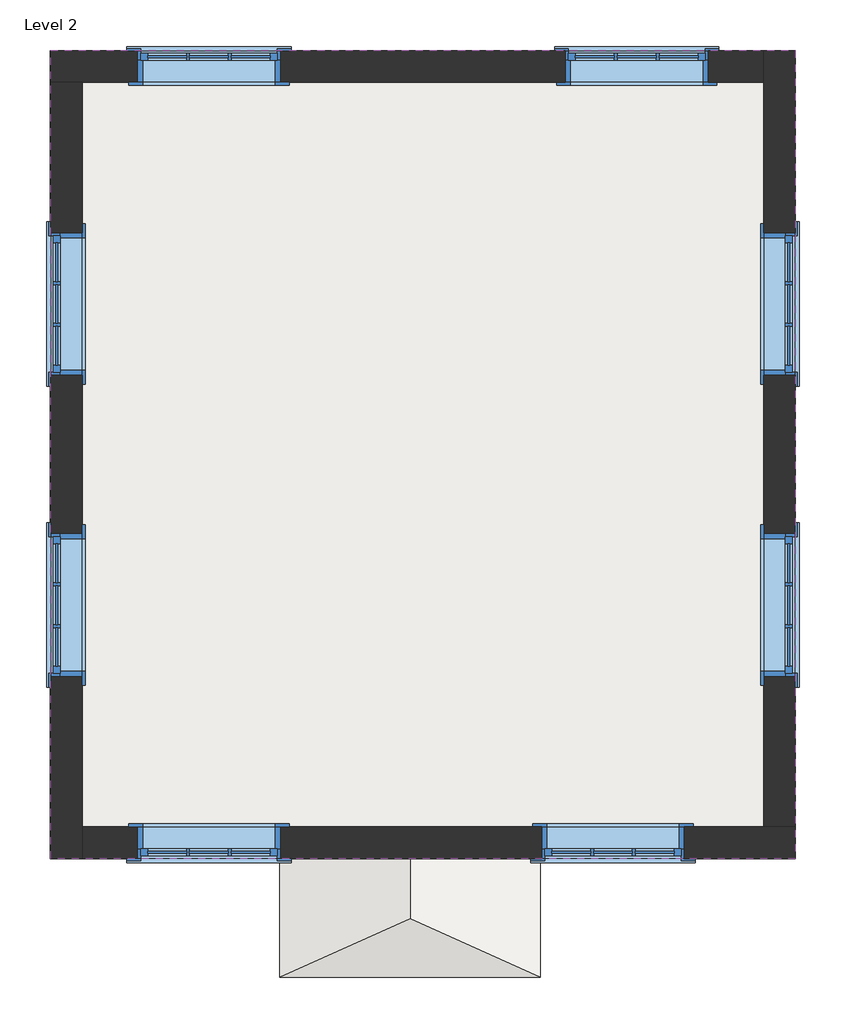
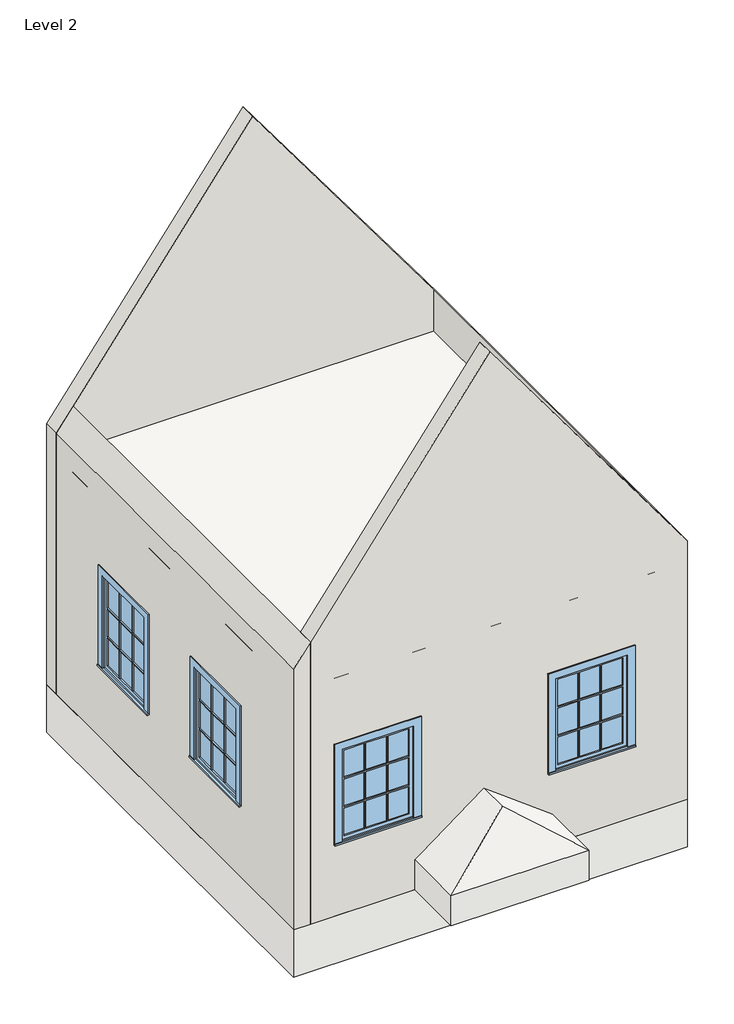
# One storey: 8 windows, 4 walls, 2 slabs, 1 roof.
"""IFC4 building model written with IfcOpenShell, lengths in millimetres."""

from ifc_helpers import new_model, si_unit, frame, origin, place, context, project, spatial, polyline, outline, extrude, faceted_brep, transform, mapped, element, save
from components import window_29c06734

model = new_model("IFC4")

# Units and contexts
model_context = context("Model", 3, world=origin())
ifc_project = project(units=[si_unit("LENGTHUNIT", "METRE", prefix="MILLI")], contexts=[model_context])

# Site, building, storey
site = spatial("IfcSite", under=ifc_project)
building = spatial("IfcBuilding", under=site)
storey = spatial("IfcBuildingStorey", under=building, Name="Level 2", Elevation=3048.0)

# Roof
placement = place(None, origin())
element("IfcRoof", 1, ObjectType="Generic - 12\"", at=placement, inside=storey, context=model_context, shape_type="Brep", body=[
    faceted_brep([(-8140.4670776, -8162.062689, 3048.0), (-8140.4670776, -7527.3100774, 3048.0), (-7305.4420776, -7527.3100774, 3674.26875), (-7305.4420776, -7787.3972655, 3674.26875), (-6470.4170776, -8162.062689, 3048.0), (-6470.4170776, -7527.3100774, 3048.0), (-8140.4670776, -7527.3100774, 3429.0), (-8140.4670776, -8289.3100774, 3429.0), (-7305.4420776, -7914.644654, 4055.26875), (-7305.4420776, -7527.3100774, 4055.26875), (-6470.4170776, -8289.3100774, 3429.0), (-6470.4170776, -7527.3100774, 3429.0), (-8140.4670776, -8289.3100774, 3048.0), (-6470.4170776, -8289.3100774, 3048.0)], [[[0, 1, 2, 3]], [[0, 3, 4]], [[5, 4, 3, 2]], [[6, 7, 8, 9]], [[7, 10, 8]], [[11, 9, 8, 10]], [[12, 7, 6, 1, 0]], [[13, 10, 7, 12]], [[5, 11, 10, 13, 4]], [[4, 13, 12, 0]], [[6, 9, 11, 5, 2, 1]]]),
])

# Slabs
element("IfcSlab", 2, ObjectType="Generic - 12\"", at=placement, inside=storey, context=model_context, shape_type="SweptSolid", body=[
    extrude(outline(polyline([(-9613.6670776, -7527.3100774), (-9613.6670776, -2345.7100774), (-4838.4670776, -2345.7100774), (-4838.4670776, -7527.3100774), (-9613.6670776, -7527.3100774)])), frame((0.0, 0.0, 2438.4), z_axis=(0.0, 0.0, 1.0), x_axis=(1.0, 0.0, 0.0)), (0.0, 0.0, 1.0), 609.6),
])
element("IfcSlab", 3, ObjectType="Generic - 12\"", at=placement, inside=storey, context=model_context, shape_type="SweptSolid", body=[
    extrude(outline(polyline([(-9610.8300594, -7527.3100774), (-9610.8300594, -2345.7100774), (-4835.6300594, -2345.7100774), (-4835.6300594, -7527.3100774), (-9610.8300594, -7527.3100774)])), frame((0.0, 0.0, 5486.4), z_axis=(0.0, 0.0, 1.0), x_axis=(1.0, 0.0, 0.0)), (0.0, 0.0, 1.0), 609.6),
])

# Walls
element("IfcWall", 4, ObjectType="Generic - 8\"", at=placement, inside=storey, context=model_context, shape_type="Brep", body=[
    faceted_brep([(-9610.8300594, -2548.9100774, 3048.0), (-9407.6300594, -2548.9100774, 3048.0), (-5038.8300594, -2548.9100774, 3048.0), (-5038.8300594, -2548.9100774, 6634.6074998), (-7233.256206, -2548.9100774, 9616.4751741), (-9407.6300594, -2548.9100774, 6661.8552999), (-9610.8300594, -2548.9100774, 6385.7396), (-5394.4300594, -2548.9100774, 5181.6), (-5394.4300594, -2548.9100774, 3962.4), (-6308.8300594, -2548.9100774, 3962.4), (-6308.8300594, -2548.9100774, 5181.6), (-8137.6300594, -2548.9100774, 5181.6), (-8137.6300594, -2548.9100774, 3962.4), (-9052.0300594, -2548.9100774, 3962.4), (-9052.0300594, -2548.9100774, 5181.6), (-9610.8300594, -2345.7100774, 3048.0), (-9610.8300594, -2345.7100774, 6385.7396), (-7233.256206, -2345.7100774, 9616.4751741), (-5038.8300594, -2345.7100774, 6634.6074998), (-5038.8300594, -2345.7100774, 3048.0), (-5394.4300594, -2345.7100774, 5181.6), (-6308.8300594, -2345.7100774, 5181.6), (-6308.8300594, -2345.7100774, 3962.4), (-5394.4300594, -2345.7100774, 3962.4), (-8137.6300594, -2345.7100774, 5181.6), (-9052.0300594, -2345.7100774, 5181.6), (-9052.0300594, -2345.7100774, 3962.4), (-8137.6300594, -2345.7100774, 3962.4)], [[[0, 1, 2, 3, 4, 5, 6], [7, 8, 9, 10], [11, 12, 13, 14]], [[15, 16, 17, 18, 19], [20, 21, 22, 23], [24, 25, 26, 27]], [[2, 1, 0, 15, 19]], [[0, 6, 16, 15]], [[3, 2, 19, 18]], [[8, 7, 20, 23]], [[9, 8, 23, 22]], [[10, 9, 22, 21]], [[7, 10, 21, 20]], [[12, 11, 24, 27]], [[13, 12, 27, 26]], [[14, 13, 26, 25]], [[11, 14, 25, 24]], [[6, 5, 4, 17, 16]], [[4, 3, 18, 17]]]),
])
element("IfcWall", 5, ObjectType="Generic - 8\"", at=placement, inside=storey, context=model_context, shape_type="Brep", body=[
    faceted_brep([(-9407.6300594, -7527.3100774, 3048.0), (-9407.6300594, -7324.1100774, 3048.0), (-9407.6300594, -2548.9100774, 3048.0), (-9407.6300594, -2548.9100774, 6661.8552999), (-9407.6300594, -7324.1100774, 6661.8552999), (-9407.6300594, -7527.3100774, 6661.8552999), (-9407.6300594, -3514.1100774, 5181.6), (-9407.6300594, -3514.1100774, 3962.4), (-9407.6300594, -4428.5100774, 3962.4), (-9407.6300594, -4428.5100774, 5181.6), (-9407.6300594, -5444.5100774, 5181.6), (-9407.6300594, -5444.5100774, 3962.4), (-9407.6300594, -6358.9100774, 3962.4), (-9407.6300594, -6358.9100774, 5181.6), (-9610.8300594, -7527.3100774, 3048.0), (-9610.8300594, -7527.3100774, 6385.7396), (-9610.8300594, -2548.9100774, 6385.7396), (-9610.8300594, -2548.9100774, 3048.0), (-9610.8300594, -3514.1100774, 5181.6), (-9610.8300594, -4428.5100774, 5181.6), (-9610.8300594, -4428.5100774, 3962.4), (-9610.8300594, -3514.1100774, 3962.4), (-9610.8300594, -5444.5100774, 5181.6), (-9610.8300594, -6358.9100774, 5181.6), (-9610.8300594, -6358.9100774, 3962.4), (-9610.8300594, -5444.5100774, 3962.4)], [[[0, 1, 2, 3, 4, 5], [6, 7, 8, 9], [10, 11, 12, 13]], [[14, 15, 16, 17], [18, 19, 20, 21], [22, 23, 24, 25]], [[2, 1, 0, 14, 17]], [[0, 5, 15, 14]], [[3, 2, 17, 16]], [[7, 6, 18, 21]], [[8, 7, 21, 20]], [[9, 8, 20, 19]], [[6, 9, 19, 18]], [[11, 10, 22, 25]], [[12, 11, 25, 24]], [[13, 12, 24, 23]], [[10, 13, 23, 22]], [[5, 4, 3, 16, 15]]]),
])
element("IfcWall", 6, ObjectType="Generic - 8\"", at=placement, inside=storey, context=model_context, shape_type="Brep", body=[
    faceted_brep([(-4835.6300594, -7324.1100774, 3048.0), (-5038.8300594, -7324.1100774, 3048.0), (-9407.6300594, -7324.1100774, 3048.0), (-9407.6300594, -7324.1100774, 6661.8552999), (-7233.256206, -7324.1100774, 9616.4751741), (-5038.8300594, -7324.1100774, 6634.6074998), (-4835.6300594, -7324.1100774, 6358.4917998), (-6461.2300594, -7324.1100774, 5181.6), (-6461.2300594, -7324.1100774, 3962.4), (-5546.8300594, -7324.1100774, 3962.4), (-5546.8300594, -7324.1100774, 5181.6), (-9052.0300594, -7324.1100774, 5181.6), (-9052.0300594, -7324.1100774, 3962.4), (-8137.6300594, -7324.1100774, 3962.4), (-8137.6300594, -7324.1100774, 5181.6), (-4835.6300594, -7527.3100774, 3048.0), (-4835.6300594, -7527.3100774, 6358.4917998), (-7233.256206, -7527.3100774, 9616.4751741), (-9407.6300594, -7527.3100774, 6661.8552999), (-9407.6300594, -7527.3100774, 3048.0), (-6461.2300594, -7527.3100774, 5181.6), (-5546.8300594, -7527.3100774, 5181.6), (-5546.8300594, -7527.3100774, 3962.4), (-6461.2300594, -7527.3100774, 3962.4), (-9052.0300594, -7527.3100774, 5181.6), (-8137.6300594, -7527.3100774, 5181.6), (-8137.6300594, -7527.3100774, 3962.4), (-9052.0300594, -7527.3100774, 3962.4)], [[[0, 1, 2, 3, 4, 5, 6], [7, 8, 9, 10], [11, 12, 13, 14]], [[15, 16, 17, 18, 19], [20, 21, 22, 23], [24, 25, 26, 27]], [[2, 1, 0, 15, 19]], [[0, 6, 16, 15]], [[3, 2, 19, 18]], [[8, 7, 20, 23]], [[9, 8, 23, 22]], [[10, 9, 22, 21]], [[7, 10, 21, 20]], [[12, 11, 24, 27]], [[13, 12, 27, 26]], [[14, 13, 26, 25]], [[11, 14, 25, 24]], [[4, 3, 18, 17]], [[6, 5, 4, 17, 16]]]),
])
element("IfcWall", 7, ObjectType="Generic - 8\"", at=placement, inside=storey, context=model_context, shape_type="Brep", body=[
    faceted_brep([(-5038.8300594, -2345.7100774, 3048.0), (-5038.8300594, -2548.9100774, 3048.0), (-5038.8300594, -7324.1100774, 3048.0), (-5038.8300594, -7324.1100774, 6634.6074998), (-5038.8300594, -2548.9100774, 6634.6074998), (-5038.8300594, -2345.7100774, 6634.6074998), (-5038.8300594, -6358.9100774, 5181.6), (-5038.8300594, -6358.9100774, 3962.4), (-5038.8300594, -5444.5100774, 3962.4), (-5038.8300594, -5444.5100774, 5181.6), (-5038.8300594, -4428.5100774, 5181.6), (-5038.8300594, -4428.5100774, 3962.4), (-5038.8300594, -3514.1100774, 3962.4), (-5038.8300594, -3514.1100774, 5181.6), (-4835.6300594, -2345.7100774, 3048.0), (-4835.6300594, -2345.7100774, 6358.4917998), (-4835.6300594, -7324.1100774, 6358.4917998), (-4835.6300594, -7324.1100774, 3048.0), (-4835.6300594, -6358.9100774, 5181.6), (-4835.6300594, -5444.5100774, 5181.6), (-4835.6300594, -5444.5100774, 3962.4), (-4835.6300594, -6358.9100774, 3962.4), (-4835.6300594, -4428.5100774, 5181.6), (-4835.6300594, -3514.1100774, 5181.6), (-4835.6300594, -3514.1100774, 3962.4), (-4835.6300594, -4428.5100774, 3962.4)], [[[0, 1, 2, 3, 4, 5], [6, 7, 8, 9], [10, 11, 12, 13]], [[14, 15, 16, 17], [18, 19, 20, 21], [22, 23, 24, 25]], [[2, 1, 0, 14, 17]], [[0, 5, 15, 14]], [[3, 2, 17, 16]], [[7, 6, 18, 21]], [[8, 7, 21, 20]], [[9, 8, 20, 19]], [[6, 9, 19, 18]], [[11, 10, 22, 25]], [[12, 11, 25, 24]], [[13, 12, 24, 23]], [[10, 13, 23, 22]], [[5, 4, 3, 16, 15]]]),
])

# Windows
window_shape = window_29c06734(model_context)
element("IfcWindow", 8, ObjectType="Casement 3x3 with Trim : 36\" x 48\"", at=placement, inside=storey, context=model_context, shape_type="MappedRepresentation", body=[
    mapped(window_shape, transform((-4937.2300594, -5901.7100774, 3048.0), x_axis=(0.0, -1.0, 0.0), y_axis=(1.0, 0.0, 0.0), z_axis=(0.0, 0.0, 1.0))),
])
element("IfcWindow", 9, ObjectType="Casement 3x3 with Trim : 36\" x 48\"", at=placement, inside=storey, context=model_context, shape_type="MappedRepresentation", body=[
    mapped(window_shape, transform((-4937.2300594, -3971.3100774, 3048.0), x_axis=(0.0, -1.0, 0.0), y_axis=(1.0, 0.0, 0.0), z_axis=(0.0, 0.0, 1.0))),
])
element("IfcWindow", 10, ObjectType="Casement 3x3 with Trim : 36\" x 48\"", at=placement, inside=storey, context=model_context, shape_type="MappedRepresentation", body=[
    mapped(window_shape, transform((-6004.0300594, -7425.7100774, 3048.0), x_axis=(-1.0, 0.0, 0.0), y_axis=(0.0, -1.0, 0.0), z_axis=(0.0, 0.0, 1.0))),
])
element("IfcWindow", 11, ObjectType="Casement 3x3 with Trim : 36\" x 48\"", at=placement, inside=storey, context=model_context, shape_type="MappedRepresentation", body=[
    mapped(window_shape, transform((-8594.8300594, -7425.7100774, 3048.0), x_axis=(-1.0, 0.0, 0.0), y_axis=(0.0, -1.0, 0.0), z_axis=(0.0, 0.0, 1.0))),
])
element("IfcWindow", 12, ObjectType="Casement 3x3 with Trim : 36\" x 48\"", at=placement, inside=storey, context=model_context, shape_type="MappedRepresentation", body=[
    mapped(window_shape, transform((-9509.2300594, -3971.3100774, 3048.0), x_axis=(0.0, 1.0, 0.0), y_axis=(-1.0, 0.0, 0.0), z_axis=(0.0, 0.0, 1.0))),
])
element("IfcWindow", 13, ObjectType="Casement 3x3 with Trim : 36\" x 48\"", at=placement, inside=storey, context=model_context, shape_type="MappedRepresentation", body=[
    mapped(window_shape, transform((-9509.2300594, -5901.7100774, 3048.0), x_axis=(0.0, 1.0, 0.0), y_axis=(-1.0, 0.0, 0.0), z_axis=(0.0, 0.0, 1.0))),
])
element("IfcWindow", 14, ObjectType="Casement 3x3 with Trim : 36\" x 48\"", at=placement, inside=storey, context=model_context, shape_type="MappedRepresentation", body=[
    mapped(window_shape, transform((-5851.6300594, -2447.3100774, 3048.0), x_axis=(1.0, 0.0, 0.0), y_axis=(0.0, 1.0, 0.0), z_axis=(0.0, 0.0, 1.0))),
])
element("IfcWindow", 15, ObjectType="Casement 3x3 with Trim : 36\" x 48\"", at=placement, inside=storey, context=model_context, shape_type="MappedRepresentation", body=[
    mapped(window_shape, transform((-8594.8300594, -2447.3100774, 3048.0), x_axis=(1.0, 0.0, 0.0), y_axis=(0.0, 1.0, 0.0), z_axis=(0.0, 0.0, 1.0))),
])

save(model, "model.ifc")

# Revit data of these elements
# Type "Generic - 12\""
#   Assembly Code = "B1020"
#   Layers, outside or top first: 1' - 0" no material (function 1)
# Type "Generic - 12\""
#   Assembly Code = "B1010"
#   Function = 0
#   Layers, outside or top first: 2' - 0" no material (function 1)
# Type "Generic - 8\""
#   Assembly Code = "B2010"
#   Layers, outside or top first: 0' - 8" no material (function 1)
# Type "Casement 3x3 with Trim : 36\" x 48\""
#   Type Mark = "10"
#   Construction Type Id = "GSP4R"
#   Assembly Code = "B2020100"
#   Analytic Construction = "1/8 in Pilkington single glazing"
#   Visual Light Transmittance = 0.9
#   Solar Heat Gain Coefficient = 0.78
#   Heat Transfer Coefficient (U) = 0.6496 BTU/(h·ft²·°F)
#   Height = 4' - 0"
#   Default Sill Height = 3' - 0"
#   Trim Projection - Ext. = 0' - 0 1/2"
#   Trim Projection - Int. = 0' - 0 3/4"
#   Trim Width - Exterior = 0' - 3 1/2"
#   Trim Width - Interior = 0' - 3 1/2"
#   Width = 3' - 0"
#   Window Inset = 0' - 0 3/4"
#   Define Thermal Properties by = 1
#   Glass Pane Material = Glass
#   Sash Material = Sash
#   Trim Exterior Material = Trim
#   Trim Interior Material = Trim
#   Wall Closure = (empty or 0)
# Element 1 (IfcRoof, "Generic - 12\"")
#   built-in parameter 1001705 = 13.3047 (stored number, unit not read)
#   built-in parameter 1001710 = 33615
#   Phase Created = New Construction
#   Materials on its faces: "Default Roof"
# Element 2 (IfcSlab, "Generic - 12\"")
#   built-in parameter 1001955 = 3.14159 (stored number, unit not read)
#   Height Offset From Level = 0' - 0"
#   Phase Created = New Construction
#   Materials on its faces: "Default Floor"
# Element 3 (IfcSlab, "Generic - 12\"")
#   built-in parameter 1001955 = 3.14159 (stored number, unit not read)
#   Height Offset From Level = 10' - 0"
#   Phase Created = New Construction
#   Materials on its faces: "Default Floor"
# Elements 4, 5, 6, 7 (IfcWall, "Generic - 8\"")
#   Top Offset = 0' - 0"
#   Base Offset = 0' - 0"
#   Unconnected Height = 10' - 0"
#   wall height = 10' - 0"
#   Phase Created = New Construction
#   Base Constraint = Level 2
#   Materials on its faces: "Default Wall"
# Element 8 (IfcWindow, "Casement 3x3 with Trim : 36\" x 48\"")
#   Mark = "17"
#   Phase Created = New Construction
#   Materials on its faces: "Sash", "Glass", "Trim"
# Element 9 (IfcWindow, "Casement 3x3 with Trim : 36\" x 48\"")
#   Mark = "18"
#   Phase Created = New Construction
#   Materials on its faces: "Sash", "Glass", "Trim"
# Element 10 (IfcWindow, "Casement 3x3 with Trim : 36\" x 48\"")
#   Mark = "19"
#   Phase Created = New Construction
#   Materials on its faces: "Sash", "Glass", "Trim"
# Element 11 (IfcWindow, "Casement 3x3 with Trim : 36\" x 48\"")
#   Mark = "20"
#   Phase Created = New Construction
#   Materials on its faces: "Sash", "Glass", "Trim"
# Element 12 (IfcWindow, "Casement 3x3 with Trim : 36\" x 48\"")
#   Mark = "21"
#   Phase Created = New Construction
#   Materials on its faces: "Sash", "Glass", "Trim"
# Element 13 (IfcWindow, "Casement 3x3 with Trim : 36\" x 48\"")
#   Mark = "22"
#   Phase Created = New Construction
#   Materials on its faces: "Sash", "Glass", "Trim"
# Element 14 (IfcWindow, "Casement 3x3 with Trim : 36\" x 48\"")
#   Mark = "23"
#   Phase Created = New Construction
#   Materials on its faces: "Sash", "Glass", "Trim"
# Element 15 (IfcWindow, "Casement 3x3 with Trim : 36\" x 48\"")
#   Mark = "24"
#   Phase Created = New Construction
#   Materials on its faces: "Sash", "Glass", "Trim"
# Materials
#   "Glass": class "Glass", colour RGB 0 128 192, transparency 0.75, Description = "Soda Lime Glass", Cost = 0
#   "Sash": class "Wood", colour RGB 224 178 126, transparency 0
#   "Trim": class "Wood", colour RGB 224 178 126, transparency 0
#   "Default Roof": colour RGB 88 101 114, transparency 0
#   "Default Floor": colour RGB 128 128 128, transparency 0
#   "Default Wall": colour RGB 128 128 128, transparency 0
